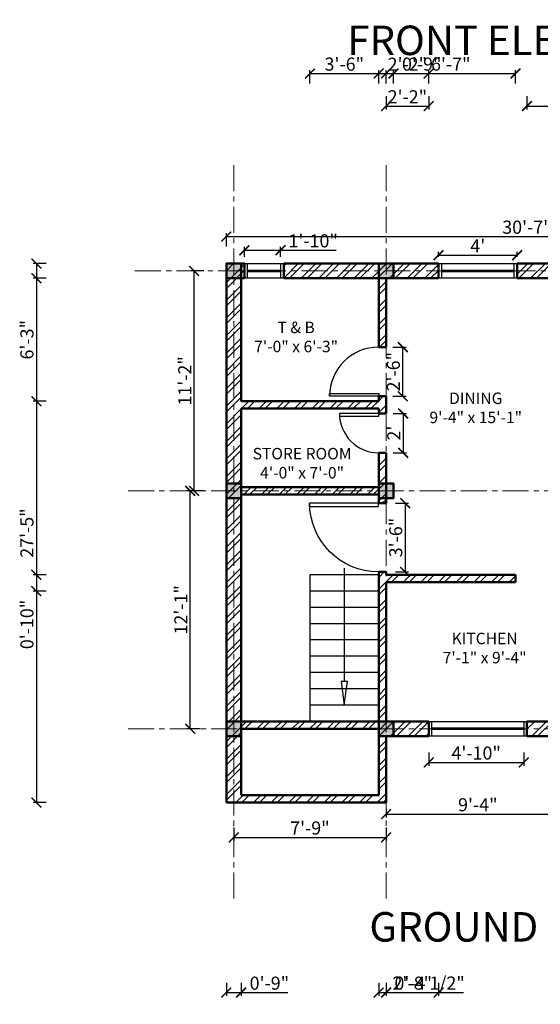
# Model space of a CAD drawing. Units: inches. Extents: x 378 to 1617, y 130 to 1256.
# Tile 1 of 5: x 390 to 708, y 130 to 731. Entities that reach past the tile are written whole.
import ezdxf

# ---------------------------------------------------------------- set-up
doc = ezdxf.new("R2010")
doc.units = ezdxf.units.IN
doc.linetypes.add('CENTER', pattern=[50.8, 31.75, -6.35, 6.35, -6.35])
for name, color, linetype, lineweight in [('A-ANNO-TEXT', 7, 'Continuous', 25), ('A-AREA-IDEN', 3, 'Continuous', 18), ('Column Hatch', 1, 'Continuous', 13), ('Columns', 241, 'Continuous', 50), ('Dimensions', 153, 'Continuous', 18), ('Doors', 2, 'Continuous', 25), ('Grid lines', 7, 'CENTER', 18), ('Stairs', 40, 'Continuous', 25), ('Wall Hatch', 11, 'Continuous', 13), ('Walls', 220, 'Continuous', 50), ('Windows', 140, 'Continuous', 25)]:
    doc.layers.add(name, color=color, linetype=linetype, lineweight=lineweight)
doc.styles.get("Standard").update_dxf_attribs({"font": 'arial.ttf'})
doc.dimstyles.new('ISO-25', dxfattribs={"dimtxt": 8, "dimasz": 6, "dimexe": 2, "dimexo": 4, "dimtad": 1, "dimdec": 0, "dimlunit": 3, "dimtxsty": 'Standard', "dimblk": 'ARCHTICK', "dimcen": 2.5, "dimadec": 0, "dimazin": 0, "dimtfac": 1, "dimtdec": 0, "dimtmove": 0, "dimatfit": 3, "dimfxl": 6, "dimfxlon": 1, "dimarcsym": 0})

# ---------------------------------------------------------------- blocks, each defined once
blk = doc.blocks.new('*U3')
for p, q in [((-30, 0), (-30, 4)), ((0, 0), (0, 4))]:
    blk.add_line(p, q)
blk.add_lwpolyline([(0, 0), (0, -30), (-1.75, -30), (-1.75, 0)], close=True)
blk.add_arc((0, 0), 30, 180, 270)
blk = doc.blocks.new('*U4')
for p, q in [((0, 0), (0, 4)), ((24, 0), (24, 4))]:
    blk.add_line(p, q)
blk.add_lwpolyline([(0, 0), (0, -24), (1.75, -24), (1.75, 0)], close=True)
blk.add_arc((0, 0), 24, 270, 0)
blk = doc.blocks.new('*U7')
for p, q in [((-36, 0), (-36, 4)), ((0, 0), (0, 4))]:
    blk.add_line(p, q)
blk.add_lwpolyline([(0, 0), (0, -36), (-1.75, -36), (-1.75, 0)], close=True)
blk.add_arc((0, 0), 36, 180, 270)
blk = doc.blocks.new('_ArchTick')
at = {"color": 0, "linetype": 'ByBlock', "const_width": 0.15}
blk.add_lwpolyline([(-0.5, -0.5), (0.5, 0.5)], dxfattribs=at)
blk = doc.blocks.new('*D8')
at = {"layer": 'Defpoints', "color": 0, "transparency": 16777216}
for p in [(521.03, 252.95), (614.03, 252.95), (614.03, 231.64)]:
    blk.add_point(p, dxfattribs=at)
at = {"layer": 'Dimensions', "color": 0, "lineweight": -2, "transparency": 16777216}
for p, q in [((521.03, 237.64), (521.03, 229.64)), ((614.03, 237.64), (614.03, 229.64)), ((521.03, 231.64), (614.03, 231.64))]:
    blk.add_line(p, q, dxfattribs=at)
at = {"layer": 'Dimensions', "color": 0, "lineweight": -2, "transparency": 16777216, "xscale": 6, "yscale": 6, "zscale": 6, "rotation": 180}
blk.add_blockref('_ArchTick', (521.03, 231.64), dxfattribs=at)
at = {"layer": 'Dimensions', "color": 0, "lineweight": -2, "transparency": 16777216, "xscale": 6, "yscale": 6, "zscale": 6}
blk.add_blockref('_ArchTick', (614.03, 231.64), dxfattribs=at)
at = {"layer": 'Dimensions', "color": 0, "transparency": 16777216, "insert": (567.53, 236.35), "char_height": 8, "attachment_point": 5}
blk.add_mtext('7\'-9"', dxfattribs=at)
blk = doc.blocks.new('*D9')
at = {"layer": 'Defpoints', "color": 0, "transparency": 16777216}
for p in [(614.03, 252.95), (726.03, 252.95), (726.03, 245.84)]:
    blk.add_point(p, dxfattribs=at)
at = {"layer": 'Dimensions', "color": 0, "lineweight": -2, "transparency": 16777216}
for p, q in [((614.03, 248.95), (614.03, 243.84)), ((726.03, 248.95), (726.03, 243.84)), ((614.03, 245.84), (726.03, 245.84))]:
    blk.add_line(p, q, dxfattribs=at)
at = {"layer": 'Dimensions', "color": 0, "lineweight": -2, "transparency": 16777216, "xscale": 6, "yscale": 6, "zscale": 6, "rotation": 180}
blk.add_blockref('_ArchTick', (614.03, 245.84), dxfattribs=at)
at = {"layer": 'Dimensions', "color": 0, "lineweight": -2, "transparency": 16777216, "xscale": 6, "yscale": 6, "zscale": 6}
blk.add_blockref('_ArchTick', (726.03, 245.84), dxfattribs=at)
at = {"layer": 'Dimensions', "color": 0, "transparency": 16777216, "insert": (670.03, 250.55), "char_height": 8, "attachment_point": 5}
blk.add_mtext('9\'-4"', dxfattribs=at)
blk = doc.blocks.new('*D11')
at = {"layer": 'Defpoints', "color": 0, "transparency": 16777216}
for p in [(494.45, 443.2), (516.53, 443.2), (516.53, 297.95)]:
    blk.add_point(p, dxfattribs=at)
at = {"layer": 'Dimensions', "color": 0, "lineweight": -2, "transparency": 16777216}
for p, q in [((500.45, 443.2), (492.45, 443.2)), ((494.45, 297.95), (494.45, 443.2)), ((500.45, 297.95), (492.45, 297.95))]:
    blk.add_line(p, q, dxfattribs=at)
at = {"layer": 'Dimensions', "color": 0, "lineweight": -2, "transparency": 16777216, "xscale": 6, "yscale": 6, "zscale": 6}
for p, rotation in [((494.45, 443.2), 90), ((494.45, 297.95), 270)]:
    blk.add_blockref('_ArchTick', p, dxfattribs=dict(at, rotation=rotation))
at = {"layer": 'Dimensions', "color": 0, "transparency": 16777216, "insert": (489.81, 370.58), "char_height": 8, "attachment_point": 5, "rotation": 90}
blk.add_mtext('12\'-1"', dxfattribs=at)
blk = doc.blocks.new('*D12')
at = {"layer": 'Defpoints', "color": 0, "transparency": 16777216}
for p in [(496.83, 577.45), (516.53, 577.45), (516.53, 443.2)]:
    blk.add_point(p, dxfattribs=at)
at = {"layer": 'Dimensions', "color": 0, "lineweight": -2, "transparency": 16777216}
for p, q in [((502.83, 577.45), (494.83, 577.45)), ((496.83, 443.2), (496.83, 577.45)), ((502.83, 443.2), (494.83, 443.2))]:
    blk.add_line(p, q, dxfattribs=at)
at = {"layer": 'Dimensions', "color": 0, "lineweight": -2, "transparency": 16777216, "xscale": 6, "yscale": 6, "zscale": 6}
for p, rotation in [((496.83, 577.45), 90), ((496.83, 443.2), 270)]:
    blk.add_blockref('_ArchTick', p, dxfattribs=dict(at, rotation=rotation))
at = {"layer": 'Dimensions', "color": 0, "transparency": 16777216, "insert": (492.19, 510.33), "char_height": 8, "attachment_point": 5, "rotation": 90}
blk.add_mtext('11\'-2"', dxfattribs=at)
blk = doc.blocks.new('*D14')
at = {"layer": 'Defpoints', "color": 0, "transparency": 16777216}
for p in [(883.53, 598.41), (516.53, 581.95), (883.53, 581.95)]:
    blk.add_point(p, dxfattribs=at)
at = {"layer": 'Dimensions', "color": 0, "lineweight": -2, "transparency": 16777216}
for p, q in [((516.53, 592.41), (516.53, 600.41)), ((516.53, 598.41), (883.53, 598.41)), ((883.53, 592.41), (883.53, 600.41))]:
    blk.add_line(p, q, dxfattribs=at)
at = {"layer": 'Dimensions', "color": 0, "lineweight": -2, "transparency": 16777216, "xscale": 6, "yscale": 6, "zscale": 6, "rotation": 180}
blk.add_blockref('_ArchTick', (516.53, 598.41), dxfattribs=at)
at = {"layer": 'Dimensions', "color": 0, "lineweight": -2, "transparency": 16777216, "xscale": 6, "yscale": 6, "zscale": 6}
blk.add_blockref('_ArchTick', (883.53, 598.41), dxfattribs=at)
at = {"layer": 'Dimensions', "color": 0, "transparency": 16777216, "insert": (700.03, 603.12), "char_height": 8, "attachment_point": 5}
blk.add_mtext('30\'-7"', dxfattribs=at)
blk = doc.blocks.new('*D24')
at = {"layer": 'Defpoints', "color": 0, "transparency": 16777216}
for p in [(549.53, 590.07), (527.53, 581.95), (549.53, 581.95)]:
    blk.add_point(p, dxfattribs=at)
at = {"layer": 'Dimensions', "color": 0, "lineweight": -2, "transparency": 16777216}
for p, q in [((527.53, 585.95), (527.53, 592.07)), ((527.53, 590.07), (549.53, 590.07)), ((549.53, 585.95), (549.53, 592.07)), ((549.53, 590.07), (583.51, 590.07))]:
    blk.add_line(p, q, dxfattribs=at)
at = {"layer": 'Dimensions', "color": 0, "lineweight": -2, "transparency": 16777216, "xscale": 6, "yscale": 6, "zscale": 6, "rotation": 180}
blk.add_blockref('_ArchTick', (527.53, 590.07), dxfattribs=at)
at = {"layer": 'Dimensions', "color": 0, "lineweight": -2, "transparency": 16777216, "xscale": 6, "yscale": 6, "zscale": 6}
blk.add_blockref('_ArchTick', (549.53, 590.07), dxfattribs=at)
at = {"layer": 'Dimensions', "color": 0, "transparency": 16777216, "insert": (569.52, 594.78), "char_height": 8, "attachment_point": 5}
blk.add_mtext('1\'-10"', dxfattribs=at)
blk = doc.blocks.new('*D25')
at = {"layer": 'Defpoints', "color": 0, "transparency": 16777216}
for p in [(694.03, 587.07), (646.03, 581.95), (694.03, 581.95)]:
    blk.add_point(p, dxfattribs=at)
at = {"layer": 'Dimensions', "color": 0, "lineweight": -2, "transparency": 16777216}
for p, q in [((646.03, 585.95), (646.03, 589.07)), ((694.03, 585.95), (694.03, 589.07)), ((646.03, 587.07), (694.03, 587.07))]:
    blk.add_line(p, q, dxfattribs=at)
at = {"layer": 'Dimensions', "color": 0, "lineweight": -2, "transparency": 16777216, "xscale": 6, "yscale": 6, "zscale": 6, "rotation": 180}
blk.add_blockref('_ArchTick', (646.03, 587.07), dxfattribs=at)
at = {"layer": 'Dimensions', "color": 0, "lineweight": -2, "transparency": 16777216, "xscale": 6, "yscale": 6, "zscale": 6}
blk.add_blockref('_ArchTick', (694.03, 587.07), dxfattribs=at)
at = {"layer": 'Dimensions', "color": 0, "transparency": 16777216, "insert": (670.03, 591.69), "char_height": 8, "attachment_point": 5}
blk.add_mtext("4'", dxfattribs=at)
blk = doc.blocks.new('*D28')
at = {"layer": 'Defpoints', "color": 0, "transparency": 16777216}
for p in [(640.03, 293.45), (698.03, 293.45), (698.03, 277.41)]:
    blk.add_point(p, dxfattribs=at)
at = {"layer": 'Dimensions', "color": 0, "lineweight": -2, "transparency": 16777216}
for p, q in [((640.03, 283.41), (640.03, 275.41)), ((698.03, 283.41), (698.03, 275.41)), ((640.03, 277.41), (698.03, 277.41))]:
    blk.add_line(p, q, dxfattribs=at)
at = {"layer": 'Dimensions', "color": 0, "lineweight": -2, "transparency": 16777216, "xscale": 6, "yscale": 6, "zscale": 6, "rotation": 180}
blk.add_blockref('_ArchTick', (640.03, 277.41), dxfattribs=at)
at = {"layer": 'Dimensions', "color": 0, "lineweight": -2, "transparency": 16777216, "xscale": 6, "yscale": 6, "zscale": 6}
blk.add_blockref('_ArchTick', (698.03, 277.41), dxfattribs=at)
at = {"layer": 'Dimensions', "color": 0, "transparency": 16777216, "insert": (669.03, 282.12), "char_height": 8, "attachment_point": 5}
blk.add_mtext('4\'-10"', dxfattribs=at)
blk = doc.blocks.new('*D31')
at = {"layer": 'Defpoints', "color": 0, "transparency": 16777216}
for p in [(611.78, 435.7), (611.69, 393.7), (625.69, 393.7)]:
    blk.add_point(p, dxfattribs=at)
at = {"layer": 'Dimensions', "color": 0, "lineweight": -2, "transparency": 16777216}
for p, q in [((619.69, 435.7), (627.69, 435.7)), ((625.69, 435.7), (625.69, 393.7)), ((619.69, 393.7), (627.69, 393.7))]:
    blk.add_line(p, q, dxfattribs=at)
at = {"layer": 'Dimensions', "color": 0, "lineweight": -2, "transparency": 16777216, "xscale": 6, "yscale": 6, "zscale": 6}
for p, rotation in [((625.69, 435.7), 90), ((625.69, 393.7), 270)]:
    blk.add_blockref('_ArchTick', p, dxfattribs=dict(at, rotation=rotation))
at = {"layer": 'Dimensions', "color": 0, "transparency": 16777216, "insert": (620.98, 414.7), "char_height": 8, "attachment_point": 5, "rotation": 90}
blk.add_mtext('3\'-6"', dxfattribs=at)
blk = doc.blocks.new('*D32')
at = {"layer": 'Defpoints', "color": 0, "transparency": 16777216}
for p in [(611.78, 490.45), (611.53, 466.45), (624.44, 466.45)]:
    blk.add_point(p, dxfattribs=at)
at = {"layer": 'Dimensions', "color": 0, "lineweight": -2, "transparency": 16777216}
for p, q in [((618.44, 490.45), (626.44, 490.45)), ((624.44, 490.45), (624.44, 466.45)), ((618.44, 466.45), (626.44, 466.45))]:
    blk.add_line(p, q, dxfattribs=at)
at = {"layer": 'Dimensions', "color": 0, "lineweight": -2, "transparency": 16777216, "xscale": 6, "yscale": 6, "zscale": 6}
for p, rotation in [((624.44, 490.45), 90), ((624.44, 466.45), 270)]:
    blk.add_blockref('_ArchTick', p, dxfattribs=dict(at, rotation=rotation))
at = {"layer": 'Dimensions', "color": 0, "transparency": 16777216, "insert": (619.8, 478.45), "char_height": 8, "attachment_point": 5, "rotation": 90}
blk.add_mtext("2'", dxfattribs=at)
blk = doc.blocks.new('*D33')
at = {"layer": 'Defpoints', "color": 0, "transparency": 16777216}
for p in [(611.78, 530.95), (624.21, 530.95), (611.78, 500.95)]:
    blk.add_point(p, dxfattribs=at)
at = {"layer": 'Dimensions', "color": 0, "lineweight": -2, "transparency": 16777216}
for p, q in [((618.21, 530.95), (626.21, 530.95)), ((624.21, 500.95), (624.21, 530.95)), ((618.21, 500.95), (626.21, 500.95))]:
    blk.add_line(p, q, dxfattribs=at)
at = {"layer": 'Dimensions', "color": 0, "lineweight": -2, "transparency": 16777216, "xscale": 6, "yscale": 6, "zscale": 6}
for p, rotation in [((624.21, 530.95), 90), ((624.21, 500.95), 270)]:
    blk.add_blockref('_ArchTick', p, dxfattribs=dict(at, rotation=rotation))
at = {"layer": 'Dimensions', "color": 0, "transparency": 16777216, "insert": (619.5, 515.95), "char_height": 8, "attachment_point": 5, "rotation": 90}
blk.add_mtext('2\'-6"', dxfattribs=at)
blk = doc.blocks.new('*D53')
at = {"layer": 'Defpoints', "color": 0, "transparency": 16777216}
for p in [(516.53, 581.95), (400.53, 252.95), (516.53, 252.95)]:
    blk.add_point(p, dxfattribs=at)
at = {"layer": 'Dimensions', "color": 0, "lineweight": -2, "transparency": 16777216}
for p, q in [((406.53, 581.95), (398.53, 581.95)), ((400.53, 581.95), (400.53, 252.95)), ((406.53, 252.95), (398.53, 252.95))]:
    blk.add_line(p, q, dxfattribs=at)
at = {"layer": 'Dimensions', "color": 0, "lineweight": -2, "transparency": 16777216, "xscale": 6, "yscale": 6, "zscale": 6}
for p, rotation in [((400.53, 581.95), 90), ((400.53, 252.95), 270)]:
    blk.add_blockref('_ArchTick', p, dxfattribs=dict(at, rotation=rotation))
at = {"layer": 'Dimensions', "color": 0, "transparency": 16777216, "insert": (395.82, 417.45), "char_height": 8, "attachment_point": 5, "rotation": 90}
blk.add_mtext('27\'-5"', dxfattribs=at)
blk = doc.blocks.new('*D54')
at = {"layer": 'Defpoints', "color": 0, "transparency": 16777216}
for p in [(516.53, 252.95), (525.53, 257.45), (525.53, 136.95)]:
    blk.add_point(p, dxfattribs=at)
at = {"layer": 'Dimensions', "color": 0, "lineweight": -2, "transparency": 16777216}
for p, q in [((516.53, 142.95), (516.53, 134.95)), ((525.53, 142.95), (525.53, 134.95)), ((516.53, 136.95), (525.53, 136.95)), ((525.53, 136.95), (554.04, 136.95))]:
    blk.add_line(p, q, dxfattribs=at)
at = {"layer": 'Dimensions', "color": 0, "lineweight": -2, "transparency": 16777216, "xscale": 6, "yscale": 6, "zscale": 6, "rotation": 180}
blk.add_blockref('_ArchTick', (516.53, 136.95), dxfattribs=at)
at = {"layer": 'Dimensions', "color": 0, "lineweight": -2, "transparency": 16777216, "xscale": 6, "yscale": 6, "zscale": 6}
blk.add_blockref('_ArchTick', (525.53, 136.95), dxfattribs=at)
at = {"layer": 'Dimensions', "color": 0, "transparency": 16777216, "insert": (542.79, 141.66), "char_height": 8, "attachment_point": 5}
blk.add_mtext('0\'-9"', dxfattribs=at)
blk = doc.blocks.new('*D55')
at = {"layer": 'Defpoints', "color": 0, "transparency": 16777216}
for p in [(609.53, 257.45), (614.03, 252.95), (614.03, 136.95)]:
    blk.add_point(p, dxfattribs=at)
at = {"layer": 'Dimensions', "color": 0, "lineweight": -2, "transparency": 16777216}
for p, q in [((609.53, 142.95), (609.53, 134.95)), ((614.03, 142.95), (614.03, 134.95)), ((609.53, 136.95), (614.03, 136.95)), ((614.03, 136.95), (661.19, 136.95))]:
    blk.add_line(p, q, dxfattribs=at)
at = {"layer": 'Dimensions', "color": 0, "lineweight": -2, "transparency": 16777216, "xscale": 6, "yscale": 6, "zscale": 6, "rotation": 180}
blk.add_blockref('_ArchTick', (609.53, 136.95), dxfattribs=at)
at = {"layer": 'Dimensions', "color": 0, "lineweight": -2, "transparency": 16777216, "xscale": 6, "yscale": 6, "zscale": 6}
blk.add_blockref('_ArchTick', (614.03, 136.95), dxfattribs=at)
at = {"layer": 'Dimensions', "color": 0, "transparency": 16777216, "insert": (640.61, 141.71), "char_height": 8, "attachment_point": 5}
blk.add_mtext('0\'-4 1/2"', dxfattribs=at)
blk = doc.blocks.new('*D56')
at = {"layer": 'Defpoints', "color": 0, "transparency": 16777216}
for p in [(618.53, 697.95), (609.53, 447.7), (618.53, 447.7)]:
    blk.add_point(p, dxfattribs=at)
at = {"layer": 'Dimensions', "color": 0, "lineweight": -2, "transparency": 16777216}
for p, q in [((609.53, 691.95), (609.53, 699.95)), ((609.53, 697.95), (618.53, 697.95)), ((618.53, 691.95), (618.53, 699.95)), ((618.53, 697.95), (647.04, 697.95))]:
    blk.add_line(p, q, dxfattribs=at)
at = {"layer": 'Dimensions', "color": 0, "lineweight": -2, "transparency": 16777216, "xscale": 6, "yscale": 6, "zscale": 6, "rotation": 180}
blk.add_blockref('_ArchTick', (609.53, 697.95), dxfattribs=at)
at = {"layer": 'Dimensions', "color": 0, "lineweight": -2, "transparency": 16777216, "xscale": 6, "yscale": 6, "zscale": 6}
blk.add_blockref('_ArchTick', (618.53, 697.95), dxfattribs=at)
at = {"layer": 'Dimensions', "color": 0, "transparency": 16777216, "insert": (635.79, 702.66), "char_height": 8, "attachment_point": 5}
blk.add_mtext('0\'-9"', dxfattribs=at)
blk = doc.blocks.new('*D57')
at = {"layer": 'Defpoints', "color": 0, "transparency": 16777216}
for p in [(614.03, 572.95), (646.03, 572.95), (646.03, 136.95)]:
    blk.add_point(p, dxfattribs=at)
at = {"layer": 'Dimensions', "color": 0, "lineweight": -2, "transparency": 16777216}
for p, q in [((614.03, 142.95), (614.03, 134.95)), ((646.03, 142.95), (646.03, 134.95)), ((614.03, 136.95), (646.03, 136.95))]:
    blk.add_line(p, q, dxfattribs=at)
at = {"layer": 'Dimensions', "color": 0, "lineweight": -2, "transparency": 16777216, "xscale": 6, "yscale": 6, "zscale": 6, "rotation": 180}
blk.add_blockref('_ArchTick', (614.03, 136.95), dxfattribs=at)
at = {"layer": 'Dimensions', "color": 0, "lineweight": -2, "transparency": 16777216, "xscale": 6, "yscale": 6, "zscale": 6}
blk.add_blockref('_ArchTick', (646.03, 136.95), dxfattribs=at)
at = {"layer": 'Dimensions', "color": 0, "transparency": 16777216, "insert": (630.03, 141.66), "char_height": 8, "attachment_point": 5}
blk.add_mtext('2\'-8"', dxfattribs=at)
blk = doc.blocks.new('*D59')
at = {"layer": 'Defpoints', "color": 0, "transparency": 16777216}
for p in [(640.03, 697.95), (614.03, 302.45), (640.03, 302.45)]:
    blk.add_point(p, dxfattribs=at)
at = {"layer": 'Dimensions', "color": 0, "lineweight": -2, "transparency": 16777216}
for p, q in [((614.03, 691.95), (614.03, 699.95)), ((614.03, 697.95), (640.03, 697.95)), ((640.03, 691.95), (640.03, 699.95))]:
    blk.add_line(p, q, dxfattribs=at)
at = {"layer": 'Dimensions', "color": 0, "lineweight": -2, "transparency": 16777216, "xscale": 6, "yscale": 6, "zscale": 6, "rotation": 180}
blk.add_blockref('_ArchTick', (614.03, 697.95), dxfattribs=at)
at = {"layer": 'Dimensions', "color": 0, "lineweight": -2, "transparency": 16777216, "xscale": 6, "yscale": 6, "zscale": 6}
blk.add_blockref('_ArchTick', (640.03, 697.95), dxfattribs=at)
at = {"layer": 'Dimensions', "color": 0, "transparency": 16777216, "insert": (627.03, 702.59), "char_height": 8, "attachment_point": 5}
blk.add_mtext('2\'-2"', dxfattribs=at)
blk = doc.blocks.new('*D61')
at = {"layer": 'Defpoints', "color": 0, "transparency": 16777216}
for p in [(693.03, 697.95), (614.03, 387.45), (693.03, 387.45)]:
    blk.add_point(p, dxfattribs=at)
at = {"layer": 'Dimensions', "color": 0, "lineweight": -2, "transparency": 16777216}
for p, q in [((614.03, 691.95), (614.03, 699.95)), ((614.03, 697.95), (693.03, 697.95)), ((693.03, 691.95), (693.03, 699.95))]:
    blk.add_line(p, q, dxfattribs=at)
at = {"layer": 'Dimensions', "color": 0, "lineweight": -2, "transparency": 16777216, "xscale": 6, "yscale": 6, "zscale": 6, "rotation": 180}
blk.add_blockref('_ArchTick', (614.03, 697.95), dxfattribs=at)
at = {"layer": 'Dimensions', "color": 0, "lineweight": -2, "transparency": 16777216, "xscale": 6, "yscale": 6, "zscale": 6}
blk.add_blockref('_ArchTick', (693.03, 697.95), dxfattribs=at)
at = {"layer": 'Dimensions', "color": 0, "transparency": 16777216, "insert": (653.53, 702.66), "char_height": 8, "attachment_point": 5}
blk.add_mtext('6\'-7"', dxfattribs=at)
blk = doc.blocks.new('*D62')
at = {"layer": 'Defpoints', "color": 0, "transparency": 16777216}
for p in [(609.53, 572.95), (400.53, 497.95), (609.53, 497.95)]:
    blk.add_point(p, dxfattribs=at)
at = {"layer": 'Dimensions', "color": 0, "lineweight": -2, "transparency": 16777216}
for p, q in [((406.53, 572.95), (398.53, 572.95)), ((400.53, 572.95), (400.53, 497.95)), ((406.53, 497.95), (398.53, 497.95))]:
    blk.add_line(p, q, dxfattribs=at)
at = {"layer": 'Dimensions', "color": 0, "lineweight": -2, "transparency": 16777216, "xscale": 6, "yscale": 6, "zscale": 6}
for p, rotation in [((400.53, 572.95), 90), ((400.53, 497.95), 270)]:
    blk.add_blockref('_ArchTick', p, dxfattribs=dict(at, rotation=rotation))
at = {"layer": 'Dimensions', "color": 0, "transparency": 16777216, "insert": (395.82, 535.45), "char_height": 8, "attachment_point": 5, "rotation": 90}
blk.add_mtext('6\'-3"', dxfattribs=at)
blk = doc.blocks.new('*D63')
at = {"layer": 'Defpoints', "color": 0, "transparency": 16777216}
for p in [(567.53, 391.95), (400.53, 382.01), (567.53, 382.01)]:
    blk.add_point(p, dxfattribs=at)
at = {"layer": 'Dimensions', "color": 0, "lineweight": -2, "transparency": 16777216}
for p, q in [((406.53, 391.95), (398.53, 391.95)), ((400.53, 391.95), (400.53, 382.01)), ((406.53, 382.01), (398.53, 382.01)), ((400.53, 382.01), (400.53, 347.27))]:
    blk.add_line(p, q, dxfattribs=at)
at = {"layer": 'Dimensions', "color": 0, "lineweight": -2, "transparency": 16777216, "xscale": 6, "yscale": 6, "zscale": 6}
for p, rotation in [((400.53, 391.95), 90), ((400.53, 382.01), 270)]:
    blk.add_blockref('_ArchTick', p, dxfattribs=dict(at, rotation=rotation))
at = {"layer": 'Dimensions', "color": 0, "transparency": 16777216, "insert": (395.82, 361.64), "char_height": 8, "attachment_point": 5, "rotation": 90}
blk.add_mtext('0\'-10"', dxfattribs=at)
blk = doc.blocks.new('*D64')
at = {"layer": 'Defpoints', "color": 0, "transparency": 16777216}
for p in [(609.53, 697.95), (567.53, 391.95), (609.53, 391.95)]:
    blk.add_point(p, dxfattribs=at)
at = {"layer": 'Dimensions', "color": 0, "lineweight": -2, "transparency": 16777216}
for p, q in [((567.53, 691.95), (567.53, 699.95)), ((567.53, 697.95), (609.53, 697.95)), ((609.53, 691.95), (609.53, 699.95))]:
    blk.add_line(p, q, dxfattribs=at)
at = {"layer": 'Dimensions', "color": 0, "lineweight": -2, "transparency": 16777216, "xscale": 6, "yscale": 6, "zscale": 6, "rotation": 180}
blk.add_blockref('_ArchTick', (567.53, 697.95), dxfattribs=at)
at = {"layer": 'Dimensions', "color": 0, "lineweight": -2, "transparency": 16777216, "xscale": 6, "yscale": 6, "zscale": 6}
blk.add_blockref('_ArchTick', (609.53, 697.95), dxfattribs=at)
at = {"layer": 'Dimensions', "color": 0, "transparency": 16777216, "insert": (588.53, 702.66), "char_height": 8, "attachment_point": 5}
blk.add_mtext('3\'-6"', dxfattribs=at)
blk = doc.blocks.new('*D81')
at = {"layer": 'Defpoints', "color": 0, "transparency": 16777216}
for p in [(640.03, 851.08), (614.03, 812.08), (640.03, 678.08)]:
    blk.add_point(p, dxfattribs=at)
at = {"layer": 'Dimensions', "color": 0, "lineweight": -2, "transparency": 16777216}
for p, q in [((614.03, 684.08), (614.03, 676.08)), ((640.03, 684.08), (640.03, 676.08)), ((614.03, 678.08), (640.03, 678.08))]:
    blk.add_line(p, q, dxfattribs=at)
at = {"layer": 'Dimensions', "color": 0, "lineweight": -2, "transparency": 16777216, "xscale": 6, "yscale": 6, "zscale": 6, "rotation": 180}
blk.add_blockref('_ArchTick', (614.03, 678.08), dxfattribs=at)
at = {"layer": 'Dimensions', "color": 0, "lineweight": -2, "transparency": 16777216, "xscale": 6, "yscale": 6, "zscale": 6}
blk.add_blockref('_ArchTick', (640.03, 678.08), dxfattribs=at)
at = {"layer": 'Dimensions', "color": 0, "transparency": 16777216, "insert": (627.03, 682.72), "char_height": 8, "attachment_point": 5}
blk.add_mtext('2\'-2"', dxfattribs=at)
blk = doc.blocks.new('*D82')
at = {"layer": 'Defpoints', "color": 0, "transparency": 16777216}
for p in [(700.03, 851.08), (733.65, 812.09), (733.65, 678.08)]:
    blk.add_point(p, dxfattribs=at)
at = {"layer": 'Dimensions', "color": 0, "lineweight": -2, "transparency": 16777216}
for p, q in [((700.03, 684.08), (700.03, 676.08)), ((733.65, 684.08), (733.65, 676.08)), ((700.03, 678.08), (733.65, 678.08)), ((733.65, 678.08), (780.95, 678.08))]:
    blk.add_line(p, q, dxfattribs=at)
at = {"layer": 'Dimensions', "color": 0, "lineweight": -2, "transparency": 16777216, "xscale": 6, "yscale": 6, "zscale": 6, "rotation": 180}
blk.add_blockref('_ArchTick', (700.03, 678.08), dxfattribs=at)
at = {"layer": 'Dimensions', "color": 0, "lineweight": -2, "transparency": 16777216, "xscale": 6, "yscale": 6, "zscale": 6}
blk.add_blockref('_ArchTick', (733.65, 678.08), dxfattribs=at)
at = {"layer": 'Dimensions', "color": 0, "transparency": 16777216, "insert": (760.3, 682.84), "char_height": 8, "attachment_point": 5}
blk.add_mtext('2\'-9 1/2"', dxfattribs=at)

msp = doc.modelspace()

# ---------------------------------------------------------------- hatches: boundary and pattern name
at = {"layer": 'Column Hatch'}
h = msp.add_hatch(color=256, dxfattribs=at)
h.dxf.hatch_style = 1
h.paths.add_polyline_path([(525.53, 581.95), (516.53, 581.95), (516.53, 572.95), (525.53, 572.95)])
h.paths.add_polyline_path([(618.53, 581.95), (609.53, 581.95), (609.53, 572.95), (618.53, 572.95)])
h.paths.add_polyline_path([(730.53, 581.95), (721.53, 581.95), (721.53, 572.95), (730.53, 572.95)])
h.paths.add_polyline_path([(883.53, 581.95), (874.53, 581.95), (874.53, 572.95), (883.53, 572.95)])
h.paths.add_polyline_path([(883.53, 447.7), (874.53, 447.7), (874.53, 438.7), (883.53, 438.7)])
h.paths.add_polyline_path([(730.53, 447.7), (721.53, 447.7), (721.53, 438.7), (730.53, 438.7)])
h.paths.add_polyline_path([(618.53, 447.7), (609.53, 447.7), (609.53, 438.7), (618.53, 438.7)])
h.paths.add_polyline_path([(525.53, 447.7), (516.53, 447.7), (516.53, 438.7), (525.53, 438.7)])
h.paths.add_polyline_path([(525.53, 302.45), (516.53, 302.45), (516.53, 293.45), (525.53, 293.45)])
h.paths.add_polyline_path([(618.53, 302.45), (609.53, 302.45), (609.53, 293.45), (618.53, 293.45)])
h.paths.add_polyline_path([(730.53, 302.45), (721.53, 302.45), (721.53, 293.45), (730.53, 293.45)])
h.paths.add_polyline_path([(883.53, 302.45), (874.53, 302.45), (874.53, 293.45), (883.53, 293.45)])
h.paths.add_polyline_path([(1125.53, 302.45), (1116.53, 302.45), (1116.53, 293.45), (1125.53, 293.45)])
h.paths.add_polyline_path([(1218.53, 302.45), (1209.53, 302.45), (1209.53, 293.45), (1218.53, 293.45)])
h.paths.add_polyline_path([(1330.53, 302.45), (1321.53, 302.45), (1321.53, 293.45), (1330.53, 293.45)])
h.paths.add_polyline_path([(1483.53, 302.45), (1474.53, 302.45), (1474.53, 293.45), (1483.53, 293.45)])
h.paths.add_polyline_path([(1483.53, 447.7), (1474.53, 447.7), (1474.53, 438.7), (1483.53, 438.7)])
h.paths.add_polyline_path([(1330.53, 447.7), (1321.53, 447.7), (1321.53, 438.7), (1330.53, 438.7)])
h.paths.add_polyline_path([(1218.53, 447.7), (1209.53, 447.7), (1209.53, 438.7), (1218.53, 438.7)])
h.paths.add_polyline_path([(1125.53, 447.7), (1116.53, 447.7), (1116.53, 438.7), (1125.53, 438.7)])
h.paths.add_polyline_path([(1125.53, 581.95), (1116.53, 581.95), (1116.53, 572.95), (1125.53, 572.95)])
h.paths.add_polyline_path([(1218.53, 581.95), (1209.53, 581.95), (1209.53, 572.95), (1218.53, 572.95)])
h.paths.add_polyline_path([(1330.53, 581.95), (1321.53, 581.95), (1321.53, 572.95), (1330.53, 572.95)])
h.paths.add_polyline_path([(1483.53, 581.95), (1474.53, 581.95), (1474.53, 572.95), (1483.53, 572.95)])
at = {"layer": 'Wall Hatch'}
h = msp.add_hatch(dxfattribs=at)
h.set_pattern_fill('ANSI32', color=256, scale=0.8)
h.paths.add_polyline_path([(525.53, 493.45), (609.53, 493.45), (609.53, 490.45), (614.03, 490.45), (614.03, 500.95), (609.53, 500.95), (609.53, 497.95), (525.53, 497.95), (525.53, 572.95), (527.53, 572.95), (527.53, 581.95), (516.53, 581.95), (516.53, 252.95), (614.03, 252.95), (614.03, 293.45), (609.53, 293.45), (609.53, 257.45), (525.53, 257.45), (525.53, 297.95), (609.53, 297.95), (609.53, 302.45), (525.53, 302.45), (525.53, 440.95), (609.53, 440.95), (609.53, 435.7), (614.03, 435.7), (614.03, 466.45), (609.53, 466.45), (609.53, 445.45), (525.53, 445.45)])
h.paths.add_polyline_path([(640.03, 302.45), (614.03, 302.45), (614.03, 387.45), (693.03, 387.45), (693.03, 391.95), (614.03, 391.95), (614.03, 393.7), (609.53, 393.7), (609.53, 293.45), (640.03, 293.45)])
h.paths.add_polyline_path([(733.53, 302.45), (730.53, 302.45), (730.53, 401.95), (726.03, 401.95), (726.03, 391.95), (723.03, 391.95), (723.03, 387.45), (726.03, 387.45), (726.03, 302.45), (700.03, 302.45), (700.03, 293.45), (733.53, 293.45)])
h.paths.add_polyline_path([(883.53, 581.95), (838.53, 581.95), (838.53, 572.95), (874.53, 572.95), (874.53, 445.45), (730.53, 445.45), (730.53, 448.45), (726.03, 448.45), (726.03, 437.95), (730.53, 437.95), (730.53, 440.95), (874.53, 440.95), (874.53, 302.45), (858.03, 302.45), (858.03, 293.45), (883.53, 293.45)])
h.paths.add_polyline_path([(730.53, 572.95), (766.53, 572.95), (766.53, 581.95), (694.03, 581.95), (694.03, 572.95), (726.03, 572.95), (726.03, 484.45), (730.53, 484.45)])
h.paths.add_polyline_path([(646.03, 581.95), (551.53, 581.95), (551.53, 572.95), (609.53, 572.95), (609.53, 530.95), (614.03, 530.95), (614.03, 572.95), (646.03, 572.95)])
h.paths.add_polyline_path([(786.03, 302.45), (769.53, 302.45), (769.53, 293.45), (786.03, 293.45)], flags=17)

# ---------------------------------------------------------------- linework, layer by layer
at = {"layer": 'Columns'}
for points in [[(516.53, 572.95), (525.53, 572.95), (525.53, 581.95), (516.53, 581.95)], [(609.53, 572.95), (618.53, 572.95), (618.53, 581.95), (609.53, 581.95)], [(516.53, 438.7), (525.53, 438.7), (525.53, 447.7), (516.53, 447.7)], [(609.53, 438.7), (618.53, 438.7), (618.53, 447.7), (609.53, 447.7)], [(516.53, 293.45), (525.53, 293.45), (525.53, 302.45), (516.53, 302.45)], [(609.53, 293.45), (618.53, 293.45), (618.53, 302.45), (609.53, 302.45)]]:
    msp.add_lwpolyline(points, close=True, dxfattribs=at)
at = {"layer": 'Grid lines', "ltscale": 0.5}
for p, q in [((521.03, 641.95), (521.03, 192.95)), ((614.03, 641.95), (614.03, 192.95)), ((460.71, 577.45), (947.71, 577.45)), ((456.53, 443.2), (943.53, 443.2)), ((456.53, 297.95), (943.53, 297.95))]:
    msp.add_line(p, q, dxfattribs=at)
at = {"layer": 'Stairs'}
for p, q in [((609.53, 391.95), (567.53, 391.95)), ((567.53, 391.95), (567.53, 302.45)), ((588.53, 395.91), (588.53, 326.75)), ((609.53, 391.95), (609.53, 302.45)), ((609.53, 382.01), (567.53, 382.01)), ((609.53, 372.06), (567.53, 372.06)), ((609.53, 362.12), (567.53, 362.12)), ((609.53, 352.17), (567.53, 352.17)), ((609.53, 342.23), (567.53, 342.23)), ((609.53, 332.28), (567.53, 332.28)), ((609.53, 322.34), (567.53, 322.34)), ((609.53, 312.4), (567.53, 312.4)), ((609.53, 302.45), (567.53, 302.45))]:
    msp.add_line(p, q, dxfattribs=at)
msp.add_lwpolyline([(586.63, 326.75), (588.53, 312.45), (590.43, 326.75)], close=True, dxfattribs=at)
at = {"layer": 'Walls'}
for p, q in [((516.53, 581.95), (527.53, 581.95)), ((516.53, 252.95), (516.53, 581.95)), ((527.53, 581.95), (527.53, 572.95)), ((551.53, 581.95), (551.53, 572.95)), ((551.53, 581.95), (646.03, 581.95)), ((646.03, 572.95), (646.03, 581.95)), ((694.03, 572.95), (694.03, 581.95)), ((694.03, 581.95), (766.53, 581.95)), ((525.53, 497.95), (525.53, 572.95)), ((525.53, 572.95), (527.53, 572.95)), ((551.53, 572.95), (609.53, 572.95)), ((609.53, 572.95), (609.53, 530.95)), ((614.03, 572.95), (614.03, 530.95)), ((614.03, 572.95), (646.03, 572.95)), ((694.03, 572.95), (726.03, 572.95)), ((609.53, 530.95), (614.03, 530.95)), ((609.53, 500.95), (614.03, 500.95)), ((609.53, 500.95), (609.53, 497.95)), ((614.03, 500.95), (614.03, 490.45)), ((609.53, 497.95), (525.53, 497.95)), ((525.53, 493.45), (525.53, 445.45)), ((609.53, 493.45), (525.53, 493.45)), ((609.53, 493.45), (609.53, 490.45)), ((609.53, 490.45), (614.03, 490.45)), ((609.53, 466.45), (614.03, 466.45)), ((609.53, 466.45), (609.53, 445.45)), ((614.03, 466.45), (614.03, 435.7)), ((609.53, 445.45), (525.53, 445.45)), ((609.53, 440.95), (525.53, 440.95)), ((525.53, 440.95), (525.53, 302.45)), ((609.53, 440.95), (609.53, 435.7)), ((609.53, 435.7), (614.03, 435.7)), ((609.53, 393.7), (614.03, 393.7)), ((609.53, 393.7), (609.53, 257.45)), ((614.03, 393.7), (614.03, 391.95)), ((614.03, 391.95), (693.03, 391.95)), ((693.03, 391.95), (693.03, 387.45)), ((614.03, 387.45), (693.03, 387.45)), ((614.03, 387.45), (614.03, 302.45)), ((609.53, 302.45), (525.53, 302.45)), ((614.03, 302.45), (640.03, 302.45)), ((640.03, 302.45), (640.03, 293.45)), ((700.03, 302.45), (700.03, 293.45)), ((700.03, 302.45), (726.03, 302.45)), ((609.53, 297.95), (525.53, 297.95)), ((525.53, 297.95), (525.53, 257.45)), ((609.53, 293.45), (640.03, 293.45)), ((614.03, 293.45), (614.03, 252.95)), ((700.03, 293.45), (733.53, 293.45)), ((614.03, 252.95), (516.53, 252.95)), ((609.53, 257.45), (525.53, 257.45))]:
    msp.add_line(p, q, dxfattribs=at)
at = {"layer": 'Windows'}
for p, q in [((527.53, 572.95), (527.53, 581.95)), ((527.53, 581.95), (551.53, 581.95)), ((529.53, 572.95), (529.53, 581.95)), ((529.53, 577.95), (549.53, 577.95)), ((549.53, 581.95), (549.53, 572.95)), ((551.53, 581.95), (551.53, 572.95)), ((646.03, 572.95), (646.03, 581.95)), ((646.03, 581.95), (694.03, 581.95)), ((648.03, 572.95), (648.03, 581.95)), ((648.03, 577.95), (692.03, 577.95)), ((692.03, 581.95), (692.03, 572.95)), ((694.03, 581.95), (694.03, 572.95)), ((551.53, 572.95), (527.53, 572.95)), ((549.53, 576.95), (529.53, 576.95)), ((694.03, 572.95), (646.03, 572.95)), ((692.03, 576.95), (648.03, 576.95)), ((640.03, 302.45), (700.03, 302.45)), ((640.03, 293.45), (640.03, 302.45)), ((642.03, 293.45), (642.03, 302.45)), ((698.03, 302.45), (698.03, 293.45)), ((700.03, 302.45), (700.03, 293.45)), ((642.03, 298.45), (698.03, 298.45)), ((698.03, 297.45), (642.03, 297.45)), ((700.03, 293.45), (640.03, 293.45))]:
    msp.add_line(p, q, dxfattribs=at)

# ---------------------------------------------------------------- block references
at = {"layer": 'Doors', "rotation": 270}
for name, p in [('*U3', (609.53, 500.95)), ('*U4', (609.53, 490.45))]:
    msp.add_blockref(name, p, dxfattribs=at)
at = {"layer": 'Doors', "xscale": -1.166666666666666, "yscale": 1.166666666666666, "zscale": 1.166666666666666, "rotation": 269.9999999999999}
msp.add_blockref('*U7', (609.36, 435.7), dxfattribs=at)

# ---------------------------------------------------------------- texts
at = {"layer": 'A-ANNO-TEXT', "char_height": 18, "attachment_point": 1}
for s, insert in [('\\pxqc;{\\fTimes New Roman|b0|i0|c0|p18;FRONT ELEVATION}', (524.62, 727.2)), ('\\pxqc;{\\fTimes New Roman|b0|i0|c0|p18;GROUND FLOOR}', (524.62, 186.07))]:
    msp.add_mtext_dynamic_manual_height_columns(s, width=345.962, gutter_width=12.5, heights=[0], dxfattribs=dict(at, insert=insert))
at = {"layer": 'A-AREA-IDEN', "char_height": 7, "attachment_point": 1}
for s, width, insert in [('\\pxqc;{\\fTimes New Roman|b0|i0|c0|p18;T & B\\P7\'-0" x 6\'-3"}', 57.8149, (530.2, 546.48)), ('\\pxqc;{\\fTimes New Roman|b0|i0|c0|p18;DINING\\P9\'-4" x 15\'-1"}', 57.8149, (639.86, 503.21)), ('\\pxqc;{\\fTimes New Roman|b0|i0|c0|p18;STORE ROOM\\P4\'-0" x 7\'-0"}', 67.3594, (529.07, 469.41)), ('\\pxqc;{\\fTimes New Roman|b0|i0|c0|p18;KITCHEN\\P7\'-1" x 9\'-4"}', 57.8149, (645.27, 356.58))]:
    msp.add_mtext_dynamic_manual_height_columns(s, width=width, gutter_width=12.5, heights=[0], dxfattribs=dict(at, insert=insert))

# ---------------------------------------------------------------- dimensions: what is measured, and where the dimension line sits
at = {"layer": 'Dimensions'}
for base, p1, p2, override, picture, middle in [((640.03, 678.08), (614.03, 812.08), (640.03, 851.08), {"dimdec": 1, "dimlfac": 1, "dimrnd": 0, "dimzin": 1, "dimdsep": 46, "dimlunit": 4, "dimfrac": 2}, '*D81', (627.03, 682.72)), ((733.65, 678.08), (700.03, 851.08), (733.65, 812.09), {"dimdec": 1, "dimlfac": 1, "dimrnd": 0, "dimzin": 1, "dimdsep": 46, "dimlunit": 4, "dimfrac": 2}, '*D82', (760.3, 682.84)), ((609.53, 697.95), (567.53, 391.95), (609.53, 391.95), {"dimdec": 1, "dimlfac": 1, "dimrnd": 0, "dimzin": 1, "dimdsep": 46, "dimlunit": 4, "dimfrac": 2}, '*D64', (588.53, 702.66)), ((618.53, 697.95), (609.53, 447.7), (618.53, 447.7), {"dimdec": 1, "dimlfac": 1, "dimrnd": 0, "dimzin": 1, "dimdsep": 46, "dimlunit": 4, "dimfrac": 2}, '*D56', (635.79, 702.66)), ((693.03, 697.95), (614.03, 387.45), (693.03, 387.45), {"dimdec": 1, "dimlfac": 1, "dimrnd": 0, "dimzin": 1, "dimdsep": 46, "dimlunit": 4, "dimfrac": 2}, '*D61', (653.53, 702.66)), ((640.03, 697.95), (614.03, 302.45), (640.03, 302.45), {"dimdec": 1, "dimlfac": 1, "dimrnd": 0, "dimzin": 1, "dimdsep": 46, "dimlunit": 4, "dimfrac": 2}, '*D59', (627.03, 702.59)), ((883.53, 598.41), (516.53, 581.95), (883.53, 581.95), {"dimclrd": 0, "dimclre": 0, "dimclrt": 0}, '*D14', (700.03, 603.12)), ((549.53, 590.07), (527.53, 581.95), (549.53, 581.95), {"dimclrd": 0, "dimclre": 0, "dimclrt": 0}, '*D24', (569.52, 594.78)), ((694.03, 587.07), (646.03, 581.95), (694.03, 581.95), {"dimclrd": 0, "dimclre": 0, "dimclrt": 0}, '*D25', (670.03, 591.69)), ((646.03, 136.95), (614.03, 572.95), (646.03, 572.95), {"dimdec": 1, "dimlfac": 1, "dimrnd": 0, "dimzin": 1, "dimdsep": 46, "dimlunit": 4, "dimfrac": 2}, '*D57', (630.03, 141.66)), ((698.03, 277.41), (640.03, 293.45), (698.03, 293.45), {"dimclrd": 0, "dimclre": 0, "dimclrt": 0}, '*D28', (669.03, 282.12)), ((525.53, 136.95), (516.53, 252.95), (525.53, 257.45), {"dimdec": 1, "dimlfac": 1, "dimrnd": 0, "dimzin": 1, "dimdsep": 46, "dimlunit": 4, "dimfrac": 2}, '*D54', (542.79, 141.66)), ((614.03, 231.64), (521.03, 252.95), (614.03, 252.95), {"dimclrd": 0, "dimclre": 0, "dimclrt": 0}, '*D8', (567.53, 236.35)), ((614.03, 136.95), (609.53, 257.45), (614.03, 252.95), {"dimdec": 1, "dimlfac": 1, "dimrnd": 0, "dimzin": 1, "dimdsep": 46, "dimlunit": 4, "dimfrac": 2}, '*D55', (640.61, 141.71)), ((726.03, 245.84), (614.03, 252.95), (726.03, 252.95), {"dimclrd": 0, "dimclre": 0, "dimclrt": 0}, '*D9', (670.03, 250.55))]:
    dim = msp.add_linear_dim(base=base, p1=p1, p2=p2, dimstyle='ISO-25', override=override, dxfattribs=at)
    dim.commit()
    dim.dimension.update_dxf_attribs({"geometry": picture, "text_midpoint": middle})
for base, p1, p2, override, picture, middle in [((400.53, 252.95), (516.53, 581.95), (516.53, 252.95), {"dimdec": 1, "dimlfac": 1, "dimrnd": 0, "dimzin": 1, "dimdsep": 46, "dimlunit": 4, "dimfrac": 2}, '*D53', (395.82, 417.45)), ((496.83, 577.45), (516.53, 443.2), (516.53, 577.45), {"dimclrd": 0, "dimclre": 0, "dimclrt": 0}, '*D12', (492.19, 510.33)), ((400.53, 497.95), (609.53, 572.95), (609.53, 497.95), {"dimdec": 1, "dimlfac": 1, "dimrnd": 0, "dimzin": 1, "dimdsep": 46, "dimlunit": 4, "dimfrac": 2}, '*D62', (395.82, 535.45)), ((400.53, 382.01), (567.53, 391.95), (567.53, 382.01), {"dimdec": 1, "dimlfac": 1, "dimrnd": 0, "dimzin": 1, "dimdsep": 46, "dimlunit": 4, "dimfrac": 2}, '*D63', (395.82, 361.64))]:
    dim = msp.add_linear_dim(base=base, p1=p1, p2=p2, angle=90, dimstyle='ISO-25', override=override, dxfattribs=at)
    dim.commit()
    dim.dimension.update_dxf_attribs({"geometry": picture, "text_midpoint": middle})
for base, p1, p2, picture, middle in [((624.21, 530.95), (611.78, 500.95), (611.78, 530.95), '*D33', (624.21, 515.95)), ((624.44, 466.45), (611.78, 490.45), (611.53, 466.45), '*D32', (624.44, 478.45)), ((494.45, 443.2), (516.53, 297.95), (516.53, 443.2), '*D11', (494.45, 370.58)), ((625.69, 393.7), (611.78, 435.7), (611.69, 393.7), '*D31', (625.69, 414.7))]:
    dim = msp.add_linear_dim(base=base, p1=p1, p2=p2, angle=90, dimstyle='ISO-25', override={"dimclrd": 0, "dimclre": 0, "dimclrt": 0}, dxfattribs=at)
    dim.commit()
    dim.dimension.update_dxf_attribs({"geometry": picture, "text_midpoint": middle, "dimtype": 160})

doc.saveas('drawing.dxf')
